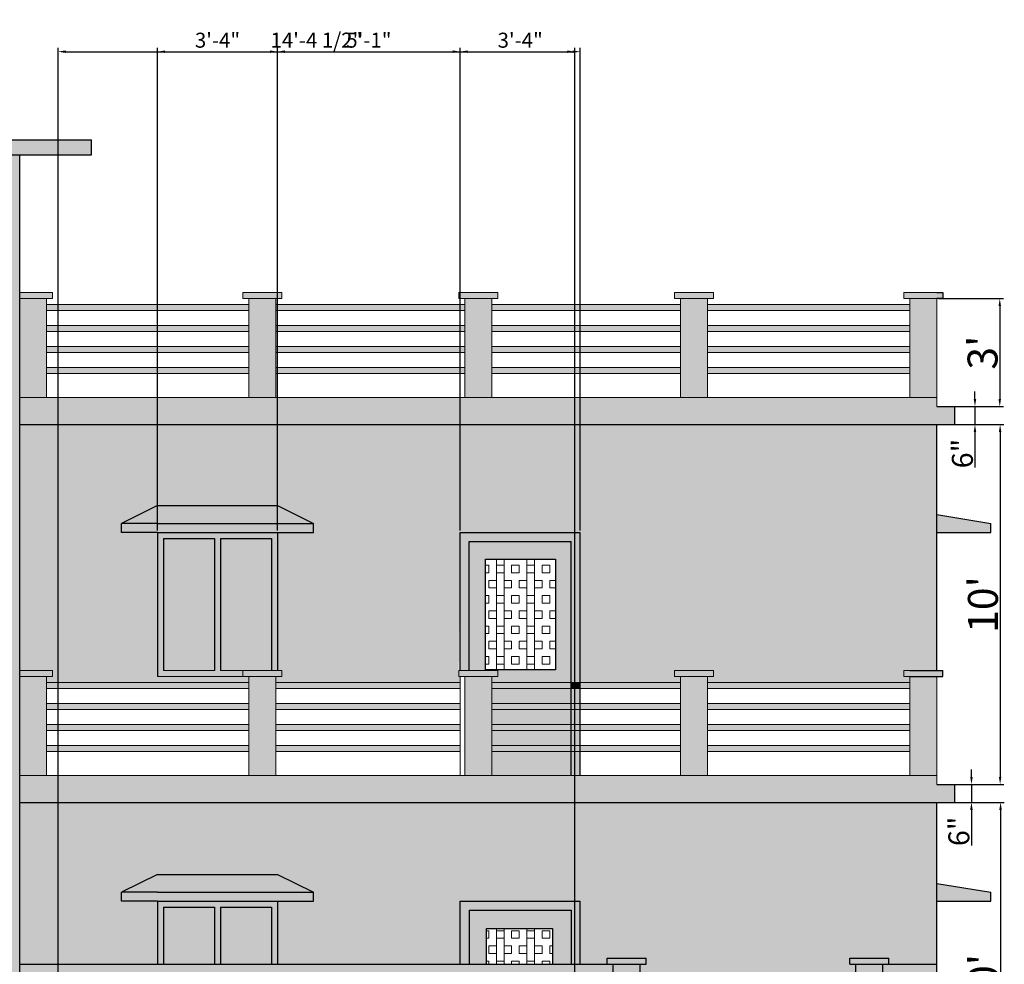
# Model space of a CAD drawing. Units: inches. Extents: x 1662 to 23131, y 1265 to 19127.
# Tile 11 of 26: x 17387 to 17716, y 7939 to 8254. Entities that reach past the tile are written whole.
import ezdxf

# ---------------------------------------------------------------- set-up
doc = ezdxf.new("R2010")
doc.units = ezdxf.units.IN
for name, color, linetype, lineweight in [('A-ANNO-DIMS', 4, 'Continuous', 18), ('A-ELEV', 7, 'Continuous', 25), ('A-ELEV-PATT', 8, 'Continuous', 13), ('A-ELEV-RAIL', 7, 'Continuous', 18), ('A-ELEV-SURF-PATT', 252, 'Continuous', 13)]:
    doc.layers.add(name, color=color, linetype=linetype, lineweight=lineweight)
doc.styles.get("Standard").update_dxf_attribs({"font": 'arial.ttf'})
doc.dimstyles.new('ISO-25', dxfattribs={"dimtxt": 5, "dimasz": 2.5, "dimexe": 1.25, "dimexo": 0.625, "dimtad": 1, "dimlunit": 3, "dimtxsty": 'Standard', "dimcen": 2.5, "dimadec": 0, "dimazin": 0, "dimtfac": 1, "dimtmove": 0, "dimatfit": 3, "dimfxl": 1, "dimarcsym": 0})

# ---------------------------------------------------------------- blocks, each defined once
blk = doc.blocks.new('*D78')
at = {"layer": 'A-ANNO-DIMS', "color": 0, "lineweight": -2, "transparency": 16777216}
for p, q in [((17693.88, 7993.16), (17715.8, 7993.16)), ((17714.55, 7990.66), (17714.55, 7875.66)), ((17693.88, 7873.16), (17715.8, 7873.16))]:
    blk.add_line(p, q, dxfattribs=at)
at = {"layer": 'A-ANNO-DIMS', "color": 0, "transparency": 16777216}
for points in [[(17714.13, 7990.66), (17714.97, 7990.66), (17714.55, 7993.16)], [(17714.13, 7875.66), (17714.97, 7875.66), (17714.55, 7873.16)]]:
    blk.add_solid(points, dxfattribs=at)
at = {"layer": 'Defpoints', "color": 0, "transparency": 16777216}
for p in [(17693.26, 7993.16), (17693.26, 7873.16), (17714.55, 7873.16)]:
    blk.add_point(p, dxfattribs=at)
at = {"layer": 'A-ANNO-DIMS', "color": 0, "transparency": 16777216, "insert": (17708.82, 7933.16), "char_height": 5, "attachment_point": 5, "rotation": 90}
blk.add_mtext("{\\H2x;10'}", dxfattribs=at)
blk = doc.blocks.new('*D79')
at = {"layer": 'A-ANNO-DIMS', "color": 0, "lineweight": -2, "transparency": 16777216}
for p, q in [((17704.84, 8001.66), (17704.84, 8004.16)), ((17699.88, 7999.16), (17706.09, 7999.16)), ((17704.84, 7999.16), (17704.84, 7993.16)), ((17699.88, 7993.16), (17706.09, 7993.16)), ((17704.84, 7990.66), (17704.84, 7978.83))]:
    blk.add_line(p, q, dxfattribs=at)
at = {"layer": 'A-ANNO-DIMS', "color": 0, "transparency": 16777216}
for points in [[(17704.42, 8001.66), (17705.26, 8001.66), (17704.84, 7999.16)], [(17704.42, 7990.66), (17705.26, 7990.66), (17704.84, 7993.16)]]:
    blk.add_solid(points, dxfattribs=at)
at = {"layer": 'Defpoints', "color": 0, "transparency": 16777216}
for p in [(17699.26, 7999.16), (17699.26, 7993.16), (17704.84, 7993.16)]:
    blk.add_point(p, dxfattribs=at)
at = {"layer": 'A-ANNO-DIMS', "color": 0, "transparency": 16777216, "insert": (17700.64, 7983.49), "char_height": 5, "attachment_point": 5, "rotation": 90}
blk.add_mtext('{\\H1.4x;6"}', dxfattribs=at)
blk = doc.blocks.new('*D80')
at = {"layer": 'A-ANNO-DIMS', "color": 0, "lineweight": -2, "transparency": 16777216}
for p, q in [((17693.88, 8119.16), (17715.65, 8119.16)), ((17714.4, 8116.66), (17714.4, 8001.66)), ((17693.88, 7999.16), (17715.65, 7999.16))]:
    blk.add_line(p, q, dxfattribs=at)
at = {"layer": 'A-ANNO-DIMS', "color": 0, "transparency": 16777216}
for points in [[(17713.98, 8116.66), (17714.82, 8116.66), (17714.4, 8119.16)], [(17713.98, 8001.66), (17714.82, 8001.66), (17714.4, 7999.16)]]:
    blk.add_solid(points, dxfattribs=at)
at = {"layer": 'Defpoints', "color": 0, "transparency": 16777216}
for p in [(17693.26, 8119.16), (17693.26, 7999.16), (17714.4, 7999.16)]:
    blk.add_point(p, dxfattribs=at)
at = {"layer": 'A-ANNO-DIMS', "color": 0, "transparency": 16777216, "insert": (17708.67, 8059.16), "char_height": 5, "attachment_point": 5, "rotation": 90}
blk.add_mtext("{\\H2x;10'}", dxfattribs=at)
blk = doc.blocks.new('*D81')
at = {"layer": 'A-ANNO-DIMS', "color": 0, "lineweight": -2, "transparency": 16777216}
for p, q in [((17706.01, 8127.66), (17706.01, 8130.16)), ((17699.88, 8125.16), (17707.26, 8125.16)), ((17706.01, 8125.16), (17706.01, 8119.16)), ((17699.88, 8119.16), (17707.26, 8119.16)), ((17706.01, 8116.66), (17706.01, 8104.83))]:
    blk.add_line(p, q, dxfattribs=at)
at = {"layer": 'A-ANNO-DIMS', "color": 0, "transparency": 16777216}
for points in [[(17705.59, 8127.66), (17706.43, 8127.66), (17706.01, 8125.16)], [(17705.59, 8116.66), (17706.43, 8116.66), (17706.01, 8119.16)]]:
    blk.add_solid(points, dxfattribs=at)
at = {"layer": 'Defpoints', "color": 0, "transparency": 16777216}
for p in [(17699.26, 8125.16), (17699.26, 8119.16), (17706.01, 8119.16)]:
    blk.add_point(p, dxfattribs=at)
at = {"layer": 'A-ANNO-DIMS', "color": 0, "transparency": 16777216, "insert": (17701.81, 8109.49), "char_height": 5, "attachment_point": 5, "rotation": 90}
blk.add_mtext('{\\H1.4x;6"}', dxfattribs=at)
blk = doc.blocks.new('*D82')
at = {"layer": 'A-ANNO-DIMS', "color": 0, "lineweight": -2, "transparency": 16777216}
for p, q in [((17693.88, 8161.16), (17715.54, 8161.16)), ((17714.29, 8158.66), (17714.29, 8127.66)), ((17693.88, 8125.16), (17715.54, 8125.16))]:
    blk.add_line(p, q, dxfattribs=at)
at = {"layer": 'A-ANNO-DIMS', "color": 0, "transparency": 16777216}
for points in [[(17713.87, 8158.66), (17714.7, 8158.66), (17714.29, 8161.16)], [(17713.87, 8127.66), (17714.7, 8127.66), (17714.29, 8125.16)]]:
    blk.add_solid(points, dxfattribs=at)
at = {"layer": 'Defpoints', "color": 0, "transparency": 16777216}
for p in [(17693.26, 8161.16), (17693.26, 8125.16), (17714.29, 8125.16)]:
    blk.add_point(p, dxfattribs=at)
at = {"layer": 'A-ANNO-DIMS', "color": 0, "transparency": 16777216, "insert": (17708.55, 8143.16), "char_height": 5, "attachment_point": 5, "rotation": 90}
blk.add_mtext("{\\H2x;3'}", dxfattribs=at)
blk = doc.blocks.new('*D234')
at = {"layer": 'A-ANNO-DIMS', "color": 0, "lineweight": -2, "transparency": 16777216}
for p, q in [((17433.26, 8083.78), (17433.26, 8244.76)), ((17435.76, 8243.51), (17470.76, 8243.51)), ((17473.26, 8083.78), (17473.26, 8244.76))]:
    blk.add_line(p, q, dxfattribs=at)
at = {"layer": 'A-ANNO-DIMS', "color": 0, "transparency": 16777216}
for points in [[(17435.76, 8243.93), (17435.76, 8243.09), (17433.26, 8243.51)], [(17470.76, 8243.93), (17470.76, 8243.09), (17473.26, 8243.51)]]:
    blk.add_solid(points, dxfattribs=at)
at = {"layer": 'Defpoints', "color": 0, "transparency": 16777216}
for p in [(17473.26, 8243.51), (17433.26, 8083.16), (17473.26, 8083.16)]:
    blk.add_point(p, dxfattribs=at)
at = {"layer": 'A-ANNO-DIMS', "color": 0, "transparency": 16777216, "insert": (17453.26, 8246.69), "char_height": 5, "attachment_point": 5}
blk.add_mtext('3\'-4"', dxfattribs=at)
blk = doc.blocks.new('*D235')
at = {"layer": 'A-ANNO-DIMS', "color": 0, "lineweight": -2, "transparency": 16777216}
for p, q in [((17473.26, 8083.78), (17473.26, 8244.76)), ((17475.76, 8243.51), (17531.76, 8243.51)), ((17534.26, 8083.78), (17534.26, 8244.76))]:
    blk.add_line(p, q, dxfattribs=at)
at = {"layer": 'A-ANNO-DIMS', "color": 0, "transparency": 16777216}
for points in [[(17475.76, 8243.93), (17475.76, 8243.09), (17473.26, 8243.51)], [(17531.76, 8243.93), (17531.76, 8243.09), (17534.26, 8243.51)]]:
    blk.add_solid(points, dxfattribs=at)
at = {"layer": 'Defpoints', "color": 0, "transparency": 16777216}
for p in [(17534.26, 8243.51), (17473.26, 8083.16), (17534.26, 8083.16)]:
    blk.add_point(p, dxfattribs=at)
at = {"layer": 'A-ANNO-DIMS', "color": 0, "transparency": 16777216, "insert": (17503.76, 8246.69), "char_height": 5, "attachment_point": 5}
blk.add_mtext('5\'-1"', dxfattribs=at)
blk = doc.blocks.new('*D236')
at = {"layer": 'A-ANNO-DIMS', "color": 0, "lineweight": -2, "transparency": 16777216}
for p, q in [((17534.26, 8083.78), (17534.26, 8244.76)), ((17536.76, 8243.51), (17571.76, 8243.51)), ((17574.26, 8083.78), (17574.26, 8244.76))]:
    blk.add_line(p, q, dxfattribs=at)
at = {"layer": 'A-ANNO-DIMS', "color": 0, "transparency": 16777216}
for points in [[(17536.76, 8243.93), (17536.76, 8243.09), (17534.26, 8243.51)], [(17571.76, 8243.93), (17571.76, 8243.09), (17574.26, 8243.51)]]:
    blk.add_solid(points, dxfattribs=at)
at = {"layer": 'Defpoints', "color": 0, "transparency": 16777216}
for p in [(17574.26, 8243.51), (17534.26, 8083.16), (17574.26, 8083.16)]:
    blk.add_point(p, dxfattribs=at)
at = {"layer": 'A-ANNO-DIMS', "color": 0, "transparency": 16777216, "insert": (17554.26, 8246.69), "char_height": 5, "attachment_point": 5}
blk.add_mtext('3\'-4"', dxfattribs=at)
blk = doc.blocks.new('*D239')
at = {"layer": 'A-ANNO-DIMS', "color": 0, "lineweight": -2, "transparency": 16777216}
for p, q in [((17400.05, 7928.94), (17400.05, 8244.76)), ((17402.55, 8243.51), (17569.96, 8243.51)), ((17572.46, 7928.94), (17572.46, 8244.76))]:
    blk.add_line(p, q, dxfattribs=at)
at = {"layer": 'A-ANNO-DIMS', "color": 0, "transparency": 16777216}
for points in [[(17402.55, 8243.93), (17402.55, 8243.09), (17400.05, 8243.51)], [(17569.96, 8243.93), (17569.96, 8243.09), (17572.46, 8243.51)]]:
    blk.add_solid(points, dxfattribs=at)
at = {"layer": 'Defpoints', "color": 0, "transparency": 16777216}
for p in [(17572.46, 8243.51), (17400.05, 7928.32), (17572.46, 7928.32)]:
    blk.add_point(p, dxfattribs=at)
at = {"layer": 'A-ANNO-DIMS', "color": 0, "transparency": 16777216, "insert": (17486.26, 8246.72), "char_height": 5, "attachment_point": 5}
blk.add_mtext('14\'-4 1/2"', dxfattribs=at)

msp = doc.modelspace()

# ---------------------------------------------------------------- hatches: boundary and pattern name
at = {"layer": 'A-ELEV-PATT'}
h = msp.add_hatch(dxfattribs=at)
h.set_pattern_fill('BOX', color=256, scale=0.4)
h.set_pattern_definition([(90, (0, 78.898), (-10.16, 6e-16), []), (90, (2.54, 78.898), (-10.16, 6e-16), []), (0, (0, 78.898), (0, 10.16), [-2.54, 2.54]), (0, (0, 81.438), (0, 10.16), [-2.54, 2.54]), (0, (0, 83.978), (0, 10.16), [2.54, -2.54]), (0, (0, 86.518), (0, 10.16), [2.54, -2.54]), (90, (5.08, 78.898), (-10.16, 6e-16), [2.54, -2.54]), (90, (7.62, 78.898), (-10.16, 6e-16), [2.54, -2.54])])
h.paths.add_polyline_path([(17566.092, 8074.225), (17542.648, 8074.225), (17542.648, 8037.316), (17566.092, 8037.316)])
h.paths.add_polyline_path([(17543.057, 7951.118), (17543.057, 7939.159), (17565.03, 7939.159), (17565.03, 7951.118)])
at = {"layer": 'A-ELEV-SURF-PATT'}
h = msp.add_hatch(color=256, dxfattribs=at)
h.dxf.hatch_style = 1
h.paths.add_polyline_path([(17263.258, 8214.159), (17263.258, 8209.159), (17411.258, 8209.159), (17411.258, 8214.159)])
h.paths.add_polyline_path([(17699.258, 8119.159), (17699.258, 8125.159), (17693.258, 8125.159), (17693.258, 8128.159), (17684.258, 8128.159), (17616.758, 8128.159), (17607.758, 8128.159), (17544.758, 8128.159), (17535.758, 8128.159), (17472.758, 8128.159), (17463.758, 8128.159), (17396.258, 8128.159), (17387.258, 8128.159), (17387.258, 8119.159)])
h.paths.add_polyline_path([(17699.258, 7993.159), (17699.258, 7999.159), (17693.258, 7999.159), (17693.258, 8002.159), (17684.258, 8002.159), (17616.758, 8002.159), (17607.758, 8002.159), (17544.758, 8002.159), (17535.758, 8002.159), (17472.758, 8002.159), (17463.758, 8002.159), (17396.258, 8002.159), (17387.258, 8002.159), (17387.258, 7993.159)])
h.paths.add_polyline_path([(17693.258, 7869.159), (17693.258, 7873.159), (17275.258, 7873.159), (17275.258, 7869.159)])
h.paths.add_polyline_path([(17396.258, 8035.159), (17398.258, 8035.159), (17398.258, 8037.159), (17396.258, 8037.159), (17387.258, 8037.159), (17387.258, 8035.159)])
h.paths.add_polyline_path([(17473.258, 8035.159), (17474.758, 8035.159), (17474.758, 8037.159), (17461.758, 8037.159), (17461.758, 8035.159)])
h.paths.add_polyline_path([(17546.758, 8037.159), (17544.758, 8037.159), (17535.758, 8037.159), (17533.758, 8037.159), (17533.758, 8035.159), (17535.758, 8035.159), (17544.758, 8035.159), (17546.758, 8035.159)])
h.paths.add_polyline_path([(17616.758, 8035.159), (17618.758, 8035.159), (17618.758, 8037.159), (17616.758, 8037.159), (17607.758, 8037.159), (17605.758, 8037.159), (17605.758, 8035.159), (17607.758, 8035.159)])
h.paths.add_polyline_path([(17695.258, 8035.159), (17695.258, 8037.159), (17684.258, 8037.159), (17682.258, 8037.159), (17682.258, 8035.159), (17684.258, 8035.159)])
h.paths.add_polyline_path([(17684.258, 8163.159), (17682.258, 8163.159), (17682.258, 8161.159), (17684.258, 8161.159), (17693.258, 8161.159), (17695.258, 8161.159), (17695.258, 8163.159), (17693.258, 8163.159)])
h.paths.add_polyline_path([(17616.758, 8161.159), (17618.758, 8161.159), (17618.758, 8163.159), (17616.758, 8163.159), (17607.758, 8163.159), (17605.758, 8163.159), (17605.758, 8161.159), (17607.758, 8161.159)])
h.paths.add_polyline_path([(17544.758, 8161.159), (17546.758, 8161.159), (17546.758, 8163.159), (17544.758, 8163.159), (17535.758, 8163.159), (17533.758, 8163.159), (17533.758, 8161.159), (17535.758, 8161.159)])
h.paths.add_polyline_path([(17463.758, 8163.159), (17461.758, 8163.159), (17461.758, 8161.159), (17463.758, 8161.159), (17472.758, 8161.159), (17474.758, 8161.159), (17474.758, 8163.159), (17472.758, 8163.159)])
h.paths.add_polyline_path([(17396.258, 8161.159), (17398.258, 8161.159), (17398.258, 8163.159), (17396.258, 8163.159), (17387.258, 8163.159), (17387.258, 8161.159)])
h.paths.add_polyline_path([(17711.258, 8083.159), (17711.258, 8086.159), (17693.258, 8089.159), (17693.258, 8083.159)])
h.paths.add_polyline_path([(17711.258, 7960.159), (17711.258, 7963.159), (17693.258, 7966.159), (17693.258, 7960.159)])
h.paths.add_polyline_path([(17263.258, 7963.159), (17263.258, 7960.159), (17275.258, 7960.159), (17275.258, 7966.159)])
h.paths.add_polyline_path([(17275.258, 8083.159), (17275.258, 8089.159), (17263.258, 8086.159), (17263.258, 8083.159)])
h = msp.add_hatch(color=256, dxfattribs=at)
h.dxf.hatch_style = 1
h.paths.add_polyline_path([(17275.258, 8209.159), (17275.258, 8041.159), (17275.258, 7873.159), (17387.258, 7873.159), (17387.258, 8209.159)])
h.paths.add_polyline_path([(17360.258, 8122.159), (17360.258, 7936.159), (17302.258, 7936.159), (17302.258, 8122.159)], flags=16)
h.paths.add_polyline_path([(17357.258, 8119.159), (17357.258, 7939.159), (17305.258, 7939.159), (17305.258, 8119.159)], flags=0)
h = msp.add_hatch(color=256, dxfattribs=at)
h.dxf.hatch_style = 1
h.paths.add_polyline_path([(17396.258, 8161.159), (17387.258, 8161.159), (17387.258, 8128.159), (17396.258, 8128.159)])
h.paths.add_polyline_path([(17463.758, 8128.159), (17472.758, 8128.159), (17472.758, 8161.159), (17463.758, 8161.159)])
h.paths.add_polyline_path([(17544.758, 8161.159), (17535.758, 8161.159), (17535.758, 8128.159), (17544.758, 8128.159)])
h.paths.add_polyline_path([(17616.758, 8161.159), (17607.758, 8161.159), (17607.758, 8128.159), (17616.758, 8128.159)])
h.paths.add_polyline_path([(17693.258, 8161.159), (17684.258, 8161.159), (17684.258, 8128.159), (17693.258, 8128.159)])
h.paths.add_polyline_path([(17396.258, 8035.159), (17387.258, 8035.159), (17387.258, 8002.159), (17396.258, 8002.159)])
h.paths.add_polyline_path([(17472.758, 8035.159), (17463.758, 8035.159), (17463.758, 8002.159), (17472.758, 8002.159)])
h.paths.add_polyline_path([(17544.758, 8035.159), (17535.758, 8035.159), (17535.758, 8002.159), (17544.758, 8002.159)])
h.paths.add_polyline_path([(17616.758, 8035.159), (17607.758, 8035.159), (17607.758, 8002.159), (17616.758, 8002.159)])
h.paths.add_polyline_path([(17684.258, 8002.159), (17693.258, 8002.159), (17693.258, 8035.159), (17684.258, 8035.159)])
h.paths.add_polyline_path([(17666.258, 7873.159), (17675.258, 7873.159), (17675.258, 7939.159), (17666.258, 7939.159)])
h.paths.add_polyline_path([(17594.258, 7939.159), (17585.258, 7939.159), (17585.258, 7873.159), (17594.258, 7873.159)])
h = msp.add_hatch(color=256, dxfattribs=at)
h.dxf.hatch_style = 1
h.paths.add_polyline_path([(17463.758, 8159.159), (17396.258, 8159.159), (17396.258, 8157.159), (17463.758, 8157.159)])
h.paths.add_polyline_path([(17463.758, 8152.159), (17396.258, 8152.159), (17396.258, 8150.159), (17463.758, 8150.159)])
h.paths.add_polyline_path([(17463.758, 8145.159), (17396.258, 8145.159), (17396.258, 8143.159), (17463.758, 8143.159)])
h.paths.add_polyline_path([(17463.758, 8138.159), (17396.258, 8138.159), (17396.258, 8136.159), (17463.758, 8136.159)])
h.paths.add_polyline_path([(17535.758, 8159.159), (17472.758, 8159.159), (17472.758, 8157.159), (17535.758, 8157.159)])
h.paths.add_polyline_path([(17535.758, 8152.159), (17472.758, 8152.159), (17472.758, 8150.159), (17535.758, 8150.159)])
h.paths.add_polyline_path([(17535.758, 8145.159), (17472.758, 8145.159), (17472.758, 8143.159), (17535.758, 8143.159)])
h.paths.add_polyline_path([(17535.758, 8138.159), (17472.758, 8138.159), (17472.758, 8136.159), (17535.758, 8136.159)])
h.paths.add_polyline_path([(17607.758, 8159.159), (17544.758, 8159.159), (17544.758, 8157.159), (17607.758, 8157.159)])
h.paths.add_polyline_path([(17607.758, 8152.159), (17544.758, 8152.159), (17544.758, 8150.159), (17607.758, 8150.159)])
h.paths.add_polyline_path([(17607.758, 8145.159), (17544.758, 8145.159), (17544.758, 8143.159), (17607.758, 8143.159)])
h.paths.add_polyline_path([(17607.758, 8138.159), (17544.758, 8138.159), (17544.758, 8136.159), (17607.758, 8136.159)])
h.paths.add_polyline_path([(17684.258, 8159.159), (17616.758, 8159.159), (17616.758, 8157.159), (17684.258, 8157.159)])
h.paths.add_polyline_path([(17684.258, 8152.159), (17616.758, 8152.159), (17616.758, 8150.159), (17684.258, 8150.159)])
h.paths.add_polyline_path([(17684.258, 8145.159), (17616.758, 8145.159), (17616.758, 8143.159), (17684.258, 8143.159)])
h.paths.add_polyline_path([(17684.258, 8138.159), (17616.758, 8138.159), (17616.758, 8136.159), (17684.258, 8136.159)])
h.paths.add_polyline_path([(17463.758, 8033.159), (17396.258, 8033.159), (17396.258, 8031.159), (17463.758, 8031.159)])
h.paths.add_polyline_path([(17463.758, 8026.159), (17396.258, 8026.159), (17396.258, 8024.159), (17463.758, 8024.159)])
h.paths.add_polyline_path([(17463.758, 8019.159), (17396.258, 8019.159), (17396.258, 8017.159), (17463.758, 8017.159)])
h.paths.add_polyline_path([(17463.758, 8012.159), (17396.258, 8012.159), (17396.258, 8010.159), (17463.758, 8010.159)])
h.paths.add_polyline_path([(17534.258, 8033.159), (17472.758, 8033.159), (17472.758, 8031.159), (17534.258, 8031.159)])
h.paths.add_polyline_path([(17534.258, 8026.159), (17472.758, 8026.159), (17472.758, 8024.159), (17534.258, 8024.159)])
h.paths.add_polyline_path([(17534.258, 8019.159), (17472.758, 8019.159), (17472.758, 8017.159), (17534.258, 8017.159)])
h.paths.add_polyline_path([(17534.258, 8012.159), (17472.758, 8012.159), (17472.758, 8010.159), (17534.258, 8010.159)])
h.paths.add_polyline_path([(17571.258, 8033.159), (17544.758, 8033.159), (17544.758, 8031.159), (17571.258, 8031.159)])
h.paths.add_polyline_path([(17571.258, 8026.159), (17544.758, 8026.159), (17544.758, 8024.159), (17571.258, 8024.159)])
h.paths.add_polyline_path([(17571.258, 8019.159), (17544.758, 8019.159), (17544.758, 8017.159), (17571.258, 8017.159)])
h.paths.add_polyline_path([(17571.258, 8012.159), (17544.758, 8012.159), (17544.758, 8010.159), (17571.258, 8010.159)])
h.paths.add_polyline_path([(17607.758, 8012.159), (17574.258, 8012.159), (17574.258, 8010.159), (17607.758, 8010.159)])
h.paths.add_polyline_path([(17607.758, 8019.159), (17574.258, 8019.159), (17574.258, 8017.159), (17607.758, 8017.159)])
h.paths.add_polyline_path([(17607.758, 8026.159), (17574.258, 8026.159), (17574.258, 8024.159), (17607.758, 8024.159)])
h.paths.add_polyline_path([(17607.758, 8033.159), (17574.258, 8033.159), (17574.258, 8031.159), (17607.758, 8031.159)])
h.paths.add_polyline_path([(17574.258, 8026.159), (17571.258, 8026.159), (17571.258, 8024.159), (17574.258, 8024.159)])
h.paths.add_polyline_path([(17574.258, 8033.159), (17571.258, 8033.159), (17571.258, 8031.159), (17574.258, 8031.159)])
h.paths.add_polyline_path([(17574.258, 8019.159), (17571.258, 8019.159), (17571.258, 8017.159), (17574.258, 8017.159)])
h.paths.add_polyline_path([(17574.258, 8012.159), (17571.258, 8012.159), (17571.258, 8010.159), (17574.258, 8010.159)])
h.paths.add_polyline_path([(17684.258, 8033.159), (17616.758, 8033.159), (17616.758, 8031.159), (17684.258, 8031.159)])
h.paths.add_polyline_path([(17684.258, 8026.159), (17616.758, 8026.159), (17616.758, 8024.159), (17684.258, 8024.159)])
h.paths.add_polyline_path([(17684.258, 8019.159), (17616.758, 8019.159), (17616.758, 8017.159), (17684.258, 8017.159)])
h.paths.add_polyline_path([(17684.258, 8012.159), (17616.758, 8012.159), (17616.758, 8010.159), (17684.258, 8010.159)])
h = msp.add_hatch(color=256, dxfattribs=at)
h.dxf.hatch_style = 1
h.paths.add_polyline_path([(17618.758, 8037.159), (17618.758, 8035.159), (17616.758, 8035.159), (17616.758, 8033.159), (17684.258, 8033.159), (17684.258, 8035.159), (17682.258, 8035.159), (17682.258, 8037.159), (17684.258, 8037.159), (17693.258, 8037.159), (17693.258, 8119.159), (17387.258, 8119.159), (17387.258, 8037.159), (17396.258, 8037.159), (17398.258, 8037.159), (17398.258, 8035.159), (17396.258, 8035.159), (17396.258, 8033.159), (17463.758, 8033.159), (17463.758, 8035.159), (17433.258, 8035.159), (17433.258, 8083.159), (17421.258, 8083.159), (17421.258, 8086.159), (17433.258, 8092.159), (17473.258, 8092.159), (17485.258, 8086.159), (17485.258, 8083.159), (17473.258, 8083.159), (17473.258, 8037.159), (17474.758, 8037.159), (17474.758, 8035.159), (17472.758, 8035.159), (17472.758, 8033.159), (17534.258, 8033.159), (17534.258, 8035.159), (17533.758, 8035.159), (17533.758, 8037.159), (17534.258, 8083.159), (17574.258, 8083.159), (17574.258, 8033.159), (17607.758, 8033.159), (17607.758, 8035.159), (17605.758, 8035.159), (17605.758, 8037.159), (17607.758, 8037.159), (17616.758, 8037.159)])
h.paths.add_polyline_path([(17387.258, 7993.159), (17387.258, 7939.159), (17433.258, 7939.159), (17433.258, 7960.159), (17421.258, 7960.159), (17421.258, 7963.159), (17433.258, 7969.159), (17473.258, 7969.159), (17485.258, 7963.159), (17485.258, 7960.159), (17473.258, 7960.159), (17473.258, 7939.159), (17534.258, 7939.159), (17534.258, 7960.159), (17574.258, 7960.159), (17574.258, 7939.159), (17583.258, 7939.159), (17583.258, 7941.159), (17596.258, 7941.159), (17596.258, 7939.159), (17594.258, 7939.159), (17594.258, 7933.159), (17666.258, 7933.159), (17666.258, 7939.159), (17664.258, 7939.159), (17664.258, 7941.159), (17677.258, 7941.159), (17677.258, 7939.159), (17693.258, 7939.159), (17693.258, 7993.159)])
h.paths.add_polyline_path([(17675.258, 7873.159), (17693.258, 7873.159), (17693.258, 7937.159), (17675.258, 7937.159)])
h.paths.add_polyline_path([(17387.258, 7873.159), (17585.258, 7873.159), (17585.258, 7937.159), (17387.258, 7937.159)])
h.paths.add_polyline_path([(17400.054, 7928.315), (17572.458, 7928.315), (17572.458, 7879.721), (17400.054, 7879.721)], flags=16)
h.paths.add_polyline_path([(17403.392, 7924.944), (17568.667, 7924.944), (17568.667, 7882.701), (17403.392, 7882.701)], flags=0)
h.paths.add_polyline_path([(17434.237, 7907.098, -1), (17410.251, 7907.098, -1)], flags=0)
h.paths.add_polyline_path([(17451.627, 7893.022, -1), (17440.234, 7893.022, -1)], flags=0)
h.paths.add_polyline_path([(17466.319, 7910.692, -1), (17448.329, 7910.692, -1)], flags=0)
h.paths.add_polyline_path([(17470.897, 7895.745, -1), (17462.194, 7895.745, -1)], flags=0)
h.paths.add_polyline_path([(17503.498, 7899.311, -1), (17477.113, 7899.311, -1)], flags=0)
h.paths.add_polyline_path([(17523.277, 7914.286, -1), (17507.105, 7914.286, -1)], flags=0)
h.paths.add_polyline_path([(17520.114, 7894.334, -1), (17509.529, 7894.334, -1)], flags=0)
h.paths.add_polyline_path([(17556.268, 7897.814, -1), (17531.682, 7897.814, -1)], flags=0)
h.paths.add_polyline_path([(17563.458, 7915.783, -1), (17553.276, 7915.783, -1)], flags=0)
h = msp.add_hatch(color=256, dxfattribs=at)
h.dxf.hatch_style = 1
h.paths.add_polyline_path([(17473.258, 8086.159), (17485.258, 8086.159), (17473.258, 8092.159), (17433.258, 8092.159), (17421.258, 8086.159), (17433.258, 8086.159)])
h.paths.add_polyline_path([(17433.258, 7969.159), (17421.258, 7963.159), (17433.258, 7963.159), (17473.258, 7963.159), (17485.258, 7963.159), (17473.258, 7969.159)])
h = msp.add_hatch(color=256, dxfattribs=at)
h.dxf.hatch_style = 1
h.paths.add_polyline_path([(17473.258, 8083.159), (17485.258, 8083.159), (17485.258, 8086.159), (17473.258, 8086.159), (17433.258, 8086.159), (17421.258, 8086.159), (17421.258, 8083.159), (17433.258, 8083.159)])
h.paths.add_polyline_path([(17433.258, 7963.159), (17421.258, 7963.159), (17421.258, 7960.159), (17433.258, 7960.159), (17473.258, 7960.159), (17485.258, 7960.159), (17485.258, 7963.159), (17473.258, 7963.159)])
h = msp.add_hatch(color=256, dxfattribs=at)
h.dxf.hatch_style = 1
h.paths.add_polyline_path([(17454.258, 8081.159), (17471.258, 8081.159), (17471.258, 8037.159), (17473.258, 8037.159), (17473.258, 8083.159), (17433.258, 8083.159), (17433.258, 8035.159), (17461.758, 8035.159), (17461.758, 8037.159), (17454.258, 8037.159)])
h.paths.add_polyline_path([(17452.258, 8037.159), (17435.258, 8037.159), (17435.258, 8081.159), (17452.258, 8081.159)], flags=16)
h.paths.add_polyline_path([(17433.258, 7939.159), (17435.258, 7939.159), (17435.258, 7958.159), (17452.258, 7958.159), (17452.258, 7939.159), (17454.258, 7939.159), (17454.258, 7958.159), (17471.258, 7958.159), (17471.258, 7939.159), (17473.258, 7939.159), (17473.258, 7960.159), (17433.258, 7960.159)])
h = msp.add_hatch(color=256, dxfattribs=at)
h.dxf.hatch_style = 1
h.paths.add_polyline_path([(17574.258, 8083.159), (17534.258, 8083.159), (17534.258, 8037.159), (17533.758, 8037.159), (17533.758, 8035.159), (17535.758, 8035.159), (17544.758, 8035.159), (17544.758, 8033.159), (17574.258, 8033.159)])
h.paths.add_polyline_path([(17542.648, 8074.225), (17566.092, 8074.225), (17566.092, 8037.316), (17542.648, 8037.316)], flags=16)
h = msp.add_hatch(color=256, dxfattribs=at)
h.dxf.hatch_style = 1
h.paths.add_polyline_path([(17574.258, 8083.159), (17534.258, 8083.159), (17534.258, 8037.159), (17533.758, 8037.159), (17533.758, 8035.159), (17535.758, 8035.159), (17544.758, 8035.159), (17544.758, 8033.159), (17574.258, 8033.159)])
h.paths.add_polyline_path([(17542.648, 8074.225), (17566.092, 8074.225), (17566.092, 8037.316), (17542.648, 8037.316)], flags=16)
h = msp.add_hatch(color=256, dxfattribs=at)
h.dxf.hatch_style = 1
h.paths.add_polyline_path([(17574.258, 8083.159), (17534.258, 8083.159), (17534.258, 8037.159), (17533.758, 8037.159), (17533.758, 8035.159), (17535.758, 8035.159), (17544.758, 8035.159), (17544.758, 8033.159), (17574.258, 8033.159)])
h.paths.add_polyline_path([(17566.092, 8037.316), (17542.648, 8037.316), (17542.648, 8074.225), (17566.092, 8074.225)], flags=16)
h = msp.add_hatch(color=256, dxfattribs=at)
h.dxf.hatch_style = 1
h.paths.add_polyline_path([(17574.258, 8083.159), (17534.258, 8083.159), (17534.258, 8037.159), (17533.758, 8037.159), (17533.758, 8035.159), (17535.758, 8035.159), (17544.758, 8035.159), (17544.758, 8033.159), (17574.258, 8033.159)])
h.paths.add_polyline_path([(17542.648, 8074.225), (17566.092, 8074.225), (17566.092, 8037.316), (17542.648, 8037.316)], flags=16)
h.paths.add_polyline_path([(17571.258, 8031.159), (17544.758, 8031.159), (17544.758, 8026.159), (17571.258, 8026.159)])
h.paths.add_polyline_path([(17571.258, 8024.159), (17544.758, 8024.159), (17544.758, 8019.159), (17571.258, 8019.159)])
h.paths.add_polyline_path([(17571.258, 8017.159), (17544.758, 8017.159), (17544.758, 8012.159), (17571.258, 8012.159)])
h.paths.add_polyline_path([(17571.258, 8010.159), (17544.758, 8010.159), (17544.758, 8002.159), (17571.258, 8002.159)])
h = msp.add_hatch(color=256, dxfattribs=at)
h.dxf.hatch_style = 1
h.paths.add_polyline_path([(17574.258, 8083.159), (17534.258, 8083.159), (17534.258, 8037.159), (17533.758, 8037.159), (17533.758, 8035.159), (17535.758, 8035.159), (17544.758, 8035.159), (17544.758, 8033.159), (17574.258, 8033.159)])
h.paths.add_polyline_path([(17566.092, 8037.316), (17542.648, 8037.316), (17542.648, 8074.225), (17566.092, 8074.225)], flags=16)
h = msp.add_hatch(color=256, dxfattribs=at)
h.dxf.hatch_style = 1
h.paths.add_polyline_path([(17534.258, 7960.159), (17534.258, 7939.159), (17537.258, 7939.159), (17537.258, 7957.159), (17571.258, 7957.159), (17571.258, 7939.159), (17574.258, 7939.159), (17574.258, 7960.159)])
h.paths.add_polyline_path([(17537.258, 8080.159), (17571.258, 8080.159), (17571.258, 8033.159), (17574.258, 8033.159), (17574.258, 8083.159), (17534.258, 8083.159), (17534.258, 8037.159), (17535.758, 8037.159), (17537.258, 8037.159)])
h = msp.add_hatch(color=256, dxfattribs=at)
h.dxf.hatch_style = 1
h.paths.add_polyline_path([(17534.258, 8037.159), (17535.758, 8037.159), (17537.258, 8037.159), (17537.258, 8080.159), (17571.258, 8080.159), (17571.258, 8033.159), (17574.258, 8033.159), (17574.258, 8083.159), (17534.258, 8083.159)])
h = msp.add_hatch(color=256, dxfattribs=at)
h.dxf.hatch_style = 1
h.paths.add_polyline_path([(17534.258, 8037.159), (17535.758, 8037.159), (17537.258, 8037.159), (17537.258, 8080.159), (17571.258, 8080.159), (17571.258, 8033.159), (17574.258, 8033.159), (17574.258, 8083.159), (17534.258, 8083.159)])
h = msp.add_hatch(color=256, dxfattribs=at)
h.dxf.hatch_style = 1
h.paths.add_polyline_path([(17435.258, 8037.159), (17452.258, 8037.159), (17452.258, 8081.159), (17435.258, 8081.159)])
h.paths.add_polyline_path([(17454.258, 8037.159), (17471.258, 8037.159), (17471.258, 8081.159), (17454.258, 8081.159)])
h.paths.add_polyline_path([(17452.258, 7958.159), (17435.258, 7958.159), (17435.258, 7939.159), (17452.258, 7939.159)])
h.paths.add_polyline_path([(17471.258, 7958.159), (17454.258, 7958.159), (17454.258, 7939.159), (17471.258, 7939.159)])
h = msp.add_hatch(color=256, dxfattribs=at)
h.dxf.hatch_style = 1
h.paths.add_polyline_path([(17544.758, 8035.159), (17546.758, 8035.159), (17546.758, 8037.159), (17544.758, 8037.159), (17535.758, 8037.159), (17533.758, 8037.159), (17533.758, 8035.159), (17535.758, 8035.159)])
h = msp.add_hatch(color=256, dxfattribs=at)
h.dxf.hatch_style = 1
h.paths.add_polyline_path([(17574.258, 8033.159), (17571.258, 8033.159), (17571.258, 8031.159), (17574.258, 8031.159)])
h.paths.add_polyline_path([(17574.258, 8031.159), (17571.258, 8031.159), (17571.258, 8026.159), (17574.258, 8026.159)])
h = msp.add_hatch(color=256, dxfattribs=at)
h.dxf.hatch_style = 1
h.paths.add_polyline_path([(17574.258, 8031.159), (17574.258, 8033.159), (17571.258, 8033.159), (17571.258, 8031.159)])
h = msp.add_hatch(color=256, dxfattribs=at)
h.dxf.hatch_style = 1
h.paths.add_polyline_path([(17571.258, 8019.159), (17574.258, 8019.159), (17574.258, 8024.159), (17571.258, 8024.159)])
h.paths.add_polyline_path([(17574.258, 8012.159), (17574.258, 8017.159), (17571.258, 8017.159), (17571.258, 8012.159)])
h.paths.add_polyline_path([(17574.258, 8010.159), (17571.258, 8010.159), (17571.258, 8002.159), (17574.258, 8002.159)])
h = msp.add_hatch(color=256, dxfattribs=at)
h.dxf.hatch_style = 1
h.paths.add_polyline_path([(17543.057, 7951.118), (17565.03, 7951.118), (17565.03, 7939.159), (17571.258, 7939.159), (17571.258, 7957.159), (17537.258, 7957.159), (17537.258, 7939.159), (17543.057, 7939.159)])
h = msp.add_hatch(color=256, dxfattribs=at)
h.dxf.hatch_style = 1
h.paths.add_polyline_path([(17596.258, 7941.159), (17583.258, 7941.159), (17583.258, 7939.159), (17596.258, 7939.159)])
h.paths.add_polyline_path([(17585.258, 7939.159), (17583.258, 7939.159), (17387.258, 7939.159), (17387.258, 7937.159), (17585.258, 7937.159)])
h.paths.add_polyline_path([(17693.258, 7939.159), (17675.258, 7939.159), (17675.258, 7937.159), (17693.258, 7937.159)])
h.paths.add_polyline_path([(17677.258, 7941.159), (17664.258, 7941.159), (17664.258, 7939.159), (17677.258, 7939.159)])

# ---------------------------------------------------------------- linework, layer by layer
at = {"layer": 'A-ELEV'}
for p, q in [((17263.258, 8214.159), (17411.258, 8214.159)), ((17411.258, 8209.159), (17411.258, 8214.159)), ((17263.258, 8209.159), (17411.258, 8209.159)), ((17387.258, 7873.159), (17387.258, 8209.159)), ((17693.258, 8163.159), (17695.258, 8163.159)), ((17695.258, 8161.159), (17693.258, 8161.159)), ((17695.258, 8163.159), (17695.258, 8161.159)), ((17693.258, 8125.159), (17699.258, 8125.159)), ((17699.258, 8119.159), (17699.258, 8125.159)), ((17387.258, 8119.159), (17699.258, 8119.159)), ((17693.258, 8037.159), (17693.258, 8119.159)), ((17433.258, 8092.159), (17421.258, 8086.159)), ((17433.258, 8092.159), (17473.258, 8092.159)), ((17473.258, 8092.159), (17485.258, 8086.159)), ((17693.258, 8089.159), (17711.258, 8086.159)), ((17433.258, 8086.159), (17421.258, 8086.159)), ((17421.258, 8083.159), (17421.258, 8086.159)), ((17433.258, 8086.159), (17473.258, 8086.159)), ((17473.258, 8086.159), (17485.258, 8086.159)), ((17485.258, 8083.159), (17485.258, 8086.159)), ((17711.258, 8083.159), (17711.258, 8086.159)), ((17433.258, 8083.159), (17421.258, 8083.159)), ((17433.258, 8083.159), (17433.258, 8035.159)), ((17433.258, 8083.159), (17473.258, 8083.159)), ((17433.258, 8083.159), (17473.258, 8083.159)), ((17473.258, 8083.159), (17473.258, 8037.159)), ((17473.258, 8083.159), (17485.258, 8083.159)), ((17534.258, 8083.159), (17574.258, 8083.159)), ((17534.258, 8037.159), (17534.258, 8083.159)), ((17574.258, 8002.159), (17574.258, 8083.159)), ((17693.258, 8083.159), (17711.258, 8083.159)), ((17435.258, 8081.159), (17435.258, 8037.159)), ((17435.258, 8081.159), (17452.258, 8081.159)), ((17452.258, 8081.159), (17452.258, 8037.159)), ((17454.258, 8081.159), (17454.258, 8037.159)), ((17454.258, 8081.159), (17471.258, 8081.159)), ((17471.258, 8081.159), (17471.258, 8037.159)), ((17537.258, 8037.159), (17537.258, 8080.159)), ((17537.258, 8080.159), (17571.258, 8080.159)), ((17571.258, 8002.159), (17571.258, 8080.159)), ((17684.258, 8037.159), (17695.258, 8037.159)), ((17695.258, 8035.159), (17695.258, 8037.159)), ((17684.258, 8035.159), (17695.258, 8035.159)), ((17693.258, 7999.159), (17699.258, 7999.159)), ((17699.258, 7993.159), (17699.258, 7999.159)), ((17387.258, 7993.159), (17699.258, 7993.159)), ((17693.258, 7821.159), (17693.258, 7993.159)), ((17433.258, 7969.159), (17421.258, 7963.159)), ((17433.258, 7969.159), (17473.258, 7969.159)), ((17473.258, 7969.159), (17485.258, 7963.159)), ((17693.258, 7966.159), (17711.258, 7963.159)), ((17433.258, 7963.159), (17421.258, 7963.159)), ((17421.258, 7960.159), (17421.258, 7963.159)), ((17433.258, 7963.159), (17473.258, 7963.159)), ((17473.258, 7963.159), (17485.258, 7963.159)), ((17485.258, 7960.159), (17485.258, 7963.159)), ((17711.258, 7960.159), (17711.258, 7963.159)), ((17433.258, 7960.159), (17421.258, 7960.159)), ((17433.258, 7960.159), (17473.258, 7960.159)), ((17433.258, 7960.159), (17473.258, 7960.159)), ((17433.258, 7960.159), (17433.258, 7939.159)), ((17435.258, 7958.159), (17452.258, 7958.159)), ((17435.258, 7958.159), (17435.258, 7939.159)), ((17452.258, 7958.159), (17452.258, 7939.159)), ((17454.258, 7958.159), (17471.258, 7958.159)), ((17454.258, 7958.159), (17454.258, 7939.159)), ((17471.258, 7958.159), (17471.258, 7939.159)), ((17473.258, 7960.159), (17473.258, 7939.159)), ((17473.258, 7960.159), (17485.258, 7960.159)), ((17534.258, 7939.159), (17534.258, 7960.159)), ((17534.258, 7960.159), (17574.258, 7960.159)), ((17574.258, 7939.159), (17574.258, 7960.159)), ((17693.258, 7960.159), (17711.258, 7960.159)), ((17537.258, 7957.159), (17571.258, 7957.159)), ((17537.258, 7957.159), (17537.258, 7939.159)), ((17571.258, 7957.159), (17571.258, 7939.159)), ((17583.258, 7941.159), (17596.258, 7941.159)), ((17583.258, 7939.159), (17583.258, 7941.159)), ((17596.258, 7939.159), (17596.258, 7941.159)), ((17664.258, 7941.159), (17677.258, 7941.159)), ((17664.258, 7939.159), (17664.258, 7941.159)), ((17677.258, 7939.159), (17677.258, 7941.159)), ((17387.258, 7939.159), (17596.258, 7939.159)), ((17585.258, 7873.159), (17585.258, 7939.159)), ((17594.258, 7873.159), (17594.258, 7939.159)), ((17664.258, 7939.159), (17693.258, 7939.159)), ((17666.258, 7873.159), (17666.258, 7939.159)), ((17675.258, 7873.159), (17675.258, 7939.159))]:
    msp.add_line(p, q, dxfattribs=at)
msp.add_lwpolyline([(17542.648, 8074.225), (17566.092, 8074.225), (17566.092, 8037.316), (17542.648, 8037.316)], close=True, dxfattribs=at)
msp.add_lwpolyline([(17543.057, 7939.159), (17543.057, 7951.118), (17565.03, 7951.118), (17565.03, 7939.159)], dxfattribs=at)
at = {"layer": 'A-ELEV-RAIL'}
for p, q in [((17387.258, 8163.159), (17396.258, 8163.159)), ((17387.258, 8161.159), (17396.258, 8161.159)), ((17398.258, 8163.159), (17396.258, 8163.159)), ((17396.258, 8128.159), (17396.258, 8161.159)), ((17396.258, 8161.159), (17398.258, 8161.159)), ((17398.258, 8161.159), (17398.258, 8163.159)), ((17461.758, 8161.159), (17461.758, 8163.159)), ((17461.758, 8163.159), (17463.758, 8163.159)), ((17463.758, 8161.159), (17461.758, 8161.159)), ((17463.758, 8163.159), (17472.758, 8163.159)), ((17463.758, 8128.159), (17463.758, 8161.159)), ((17463.758, 8161.159), (17472.758, 8161.159)), ((17472.758, 8163.159), (17474.758, 8163.159)), ((17472.758, 8128.159), (17472.758, 8161.159)), ((17474.758, 8161.159), (17472.758, 8161.159)), ((17474.758, 8163.159), (17474.758, 8161.159)), ((17533.758, 8161.159), (17533.758, 8163.159)), ((17533.758, 8163.159), (17535.758, 8163.159)), ((17535.758, 8161.159), (17533.758, 8161.159)), ((17535.758, 8163.159), (17544.758, 8163.159)), ((17535.758, 8128.159), (17535.758, 8161.159)), ((17535.758, 8161.159), (17544.758, 8161.159)), ((17544.758, 8163.159), (17546.758, 8163.159)), ((17544.758, 8128.159), (17544.758, 8161.159)), ((17546.758, 8161.159), (17544.758, 8161.159)), ((17546.758, 8163.159), (17546.758, 8161.159)), ((17607.758, 8163.159), (17605.758, 8163.159)), ((17605.758, 8163.159), (17605.758, 8161.159)), ((17605.758, 8161.159), (17607.758, 8161.159)), ((17607.758, 8163.159), (17616.758, 8163.159)), ((17607.758, 8128.159), (17607.758, 8161.159)), ((17607.758, 8161.159), (17616.758, 8161.159)), ((17618.758, 8163.159), (17616.758, 8163.159)), ((17616.758, 8128.159), (17616.758, 8161.159)), ((17616.758, 8161.159), (17618.758, 8161.159)), ((17618.758, 8161.159), (17618.758, 8163.159)), ((17682.258, 8161.159), (17682.258, 8163.159)), ((17682.258, 8163.159), (17684.258, 8163.159)), ((17684.258, 8161.159), (17682.258, 8161.159)), ((17684.258, 8163.159), (17693.258, 8163.159)), ((17684.258, 8128.159), (17684.258, 8161.159)), ((17684.258, 8161.159), (17693.258, 8161.159)), ((17693.258, 8125.159), (17693.258, 8161.159)), ((17396.258, 8159.159), (17463.758, 8159.159)), ((17472.758, 8159.159), (17535.758, 8159.159)), ((17544.758, 8159.159), (17607.758, 8159.159)), ((17616.758, 8159.159), (17684.258, 8159.159)), ((17396.258, 8157.159), (17463.758, 8157.159)), ((17472.758, 8157.159), (17535.758, 8157.159)), ((17544.758, 8157.159), (17607.758, 8157.159)), ((17616.758, 8157.159), (17684.258, 8157.159)), ((17396.258, 8152.159), (17463.758, 8152.159)), ((17472.758, 8152.159), (17535.758, 8152.159)), ((17544.758, 8152.159), (17607.758, 8152.159)), ((17616.758, 8152.159), (17684.258, 8152.159)), ((17396.258, 8150.159), (17463.758, 8150.159)), ((17472.758, 8150.159), (17535.758, 8150.159)), ((17544.758, 8150.159), (17607.758, 8150.159)), ((17616.758, 8150.159), (17684.258, 8150.159)), ((17396.258, 8145.159), (17463.758, 8145.159)), ((17472.758, 8145.159), (17535.758, 8145.159)), ((17544.758, 8145.159), (17607.758, 8145.159)), ((17616.758, 8145.159), (17684.258, 8145.159)), ((17396.258, 8143.159), (17463.758, 8143.159)), ((17472.758, 8143.159), (17535.758, 8143.159)), ((17544.758, 8143.159), (17607.758, 8143.159)), ((17616.758, 8143.159), (17684.258, 8143.159)), ((17396.258, 8138.159), (17463.758, 8138.159)), ((17472.758, 8138.159), (17535.758, 8138.159)), ((17544.758, 8138.159), (17607.758, 8138.159)), ((17616.758, 8138.159), (17684.258, 8138.159)), ((17396.258, 8136.159), (17463.758, 8136.159)), ((17472.758, 8136.159), (17535.758, 8136.159)), ((17544.758, 8136.159), (17607.758, 8136.159)), ((17616.758, 8136.159), (17684.258, 8136.159)), ((17396.258, 8128.159), (17387.258, 8128.159)), ((17396.258, 8128.159), (17463.758, 8128.159)), ((17463.758, 8128.159), (17472.758, 8128.159)), ((17472.758, 8128.159), (17535.758, 8128.159)), ((17535.758, 8128.159), (17544.758, 8128.159)), ((17544.758, 8128.159), (17607.758, 8128.159)), ((17544.758, 8128.159), (17607.758, 8128.159)), ((17607.758, 8128.159), (17616.758, 8128.159)), ((17616.758, 8128.159), (17684.258, 8128.159)), ((17684.258, 8128.159), (17693.258, 8128.159)), ((17396.258, 8037.159), (17387.258, 8037.159)), ((17398.258, 8037.159), (17396.258, 8037.159)), ((17398.258, 8035.159), (17398.258, 8037.159)), ((17435.258, 8037.159), (17452.258, 8037.159)), ((17454.258, 8037.159), (17471.258, 8037.159)), ((17474.758, 8037.159), (17461.758, 8037.159)), ((17461.758, 8037.159), (17461.758, 8035.159)), ((17474.758, 8035.159), (17474.758, 8037.159)), ((17535.758, 8037.159), (17533.758, 8037.159)), ((17533.758, 8037.159), (17533.758, 8035.159)), ((17535.758, 8037.159), (17544.758, 8037.159)), ((17546.758, 8037.159), (17544.758, 8037.159)), ((17546.758, 8035.159), (17546.758, 8037.159)), ((17607.758, 8037.159), (17605.758, 8037.159)), ((17605.758, 8037.159), (17605.758, 8035.159)), ((17607.758, 8037.159), (17616.758, 8037.159)), ((17618.758, 8037.159), (17616.758, 8037.159)), ((17618.758, 8035.159), (17618.758, 8037.159)), ((17682.258, 8035.159), (17682.258, 8037.159)), ((17682.258, 8037.159), (17684.258, 8037.159)), ((17396.258, 8035.159), (17387.258, 8035.159)), ((17396.258, 8002.159), (17396.258, 8035.159)), ((17396.258, 8035.159), (17398.258, 8035.159)), ((17396.258, 8033.159), (17463.758, 8033.159)), ((17433.258, 8035.159), (17473.258, 8035.159)), ((17461.758, 8035.159), (17463.758, 8035.159)), ((17463.758, 8002.159), (17463.758, 8035.159)), ((17472.758, 8002.159), (17472.758, 8035.159)), ((17472.758, 8035.159), (17474.758, 8035.159)), ((17472.758, 8033.159), (17534.258, 8033.159)), ((17533.758, 8035.159), (17535.758, 8035.159)), ((17534.258, 8002.159), (17534.258, 8035.159)), ((17535.758, 8002.159), (17535.758, 8035.159)), ((17535.758, 8035.159), (17544.758, 8035.159)), ((17544.758, 8002.159), (17544.758, 8035.159)), ((17544.758, 8035.159), (17546.758, 8035.159)), ((17544.758, 8033.159), (17607.758, 8033.159)), ((17605.758, 8035.159), (17607.758, 8035.159)), ((17607.758, 8002.159), (17607.758, 8035.159)), ((17607.758, 8035.159), (17616.758, 8035.159)), ((17616.758, 8002.159), (17616.758, 8035.159)), ((17616.758, 8035.159), (17618.758, 8035.159)), ((17616.758, 8033.159), (17684.258, 8033.159)), ((17684.258, 8035.159), (17682.258, 8035.159)), ((17684.258, 8002.159), (17684.258, 8035.159)), ((17693.258, 7999.159), (17693.258, 8035.159)), ((17396.258, 8031.159), (17463.758, 8031.159)), ((17472.758, 8031.159), (17534.258, 8031.159)), ((17544.758, 8031.159), (17607.758, 8031.159)), ((17616.758, 8031.159), (17684.258, 8031.159)), ((17396.258, 8026.159), (17463.758, 8026.159)), ((17396.258, 8024.159), (17463.758, 8024.159)), ((17472.758, 8026.159), (17534.258, 8026.159)), ((17472.758, 8024.159), (17534.258, 8024.159)), ((17544.758, 8026.159), (17607.758, 8026.159)), ((17544.758, 8024.159), (17607.758, 8024.159)), ((17616.758, 8026.159), (17684.258, 8026.159)), ((17616.758, 8024.159), (17684.258, 8024.159)), ((17396.258, 8019.159), (17463.758, 8019.159)), ((17396.258, 8017.159), (17463.758, 8017.159)), ((17472.758, 8019.159), (17534.258, 8019.159)), ((17472.758, 8017.159), (17534.258, 8017.159)), ((17544.758, 8019.159), (17607.758, 8019.159)), ((17544.758, 8017.159), (17607.758, 8017.159)), ((17616.758, 8019.159), (17684.258, 8019.159)), ((17616.758, 8017.159), (17684.258, 8017.159)), ((17396.258, 8012.159), (17463.758, 8012.159)), ((17396.258, 8010.159), (17463.758, 8010.159)), ((17472.758, 8012.159), (17534.258, 8012.159)), ((17472.758, 8010.159), (17534.258, 8010.159)), ((17544.758, 8012.159), (17607.758, 8012.159)), ((17544.758, 8010.159), (17607.758, 8010.159)), ((17616.758, 8012.159), (17684.258, 8012.159)), ((17616.758, 8010.159), (17684.258, 8010.159)), ((17396.258, 8002.159), (17387.258, 8002.159)), ((17396.258, 8002.159), (17463.758, 8002.159)), ((17463.758, 8002.159), (17472.758, 8002.159)), ((17472.758, 8002.159), (17535.758, 8002.159)), ((17535.758, 8002.159), (17544.758, 8002.159)), ((17544.758, 8002.159), (17607.758, 8002.159)), ((17607.758, 8002.159), (17616.758, 8002.159)), ((17616.758, 8002.159), (17684.258, 8002.159)), ((17684.258, 8002.159), (17693.258, 8002.159))]:
    msp.add_line(p, q, dxfattribs=at)

# ---------------------------------------------------------------- dimensions: what is measured, and where the dimension line sits
at = {"layer": 'A-ANNO-DIMS'}
for base, p1, p2, picture, middle in [((17572.458, 8243.509), (17400.054, 7928.315), (17572.458, 7928.315), '*D239', (17486.256, 8246.72)), ((17473.258, 8243.509), (17433.258, 8083.159), (17473.258, 8083.159), '*D234', (17453.258, 8246.689)), ((17534.258, 8243.509), (17473.258, 8083.159), (17534.258, 8083.159), '*D235', (17503.758, 8246.687)), ((17574.258, 8243.509), (17534.258, 8083.159), (17574.258, 8083.159), '*D236', (17554.258, 8246.689))]:
    dim = msp.add_linear_dim(base=base, p1=p1, p2=p2, dimstyle='ISO-25', override={"dimdec": 1, "dimlfac": 1, "dimrnd": 0, "dimzin": 1, "dimdsep": 46, "dimlunit": 4, "dimfrac": 2}, dxfattribs=at)
    dim.commit()
    dim.dimension.update_dxf_attribs({"geometry": picture, "text_midpoint": middle})
for base, p1, p2, text, picture, middle in [((17714.287, 8125.159), (17693.258, 8161.159), (17693.258, 8125.159), '{\\H2x;<>}', '*D82', (17708.553, 8143.159)), ((17706.011, 8119.159), (17699.258, 8125.159), (17699.258, 8119.159), '{\\H1.4x;<>}', '*D81', (17701.812, 8109.492)), ((17714.401, 7999.159), (17693.258, 8119.159), (17693.258, 7999.159), '{\\H2x;<>}', '*D80', (17708.67, 8059.159)), ((17704.842, 7993.159), (17699.258, 7999.159), (17699.258, 7993.159), '{\\H1.4x;<>}', '*D79', (17700.643, 7983.492)), ((17714.55, 7873.159), (17693.258, 7993.159), (17693.258, 7873.159), '{\\H2x;<>}', '*D78', (17708.819, 7933.159))]:
    dim = msp.add_linear_dim(base=base, p1=p1, p2=p2, angle=90, text=text, dimstyle='ISO-25', override={"dimclrd": 0, "dimclre": 0, "dimclrt": 0}, dxfattribs=at)
    dim.commit()
    dim.dimension.update_dxf_attribs({"geometry": picture, "text_midpoint": middle})

doc.saveas('drawing.dxf')
